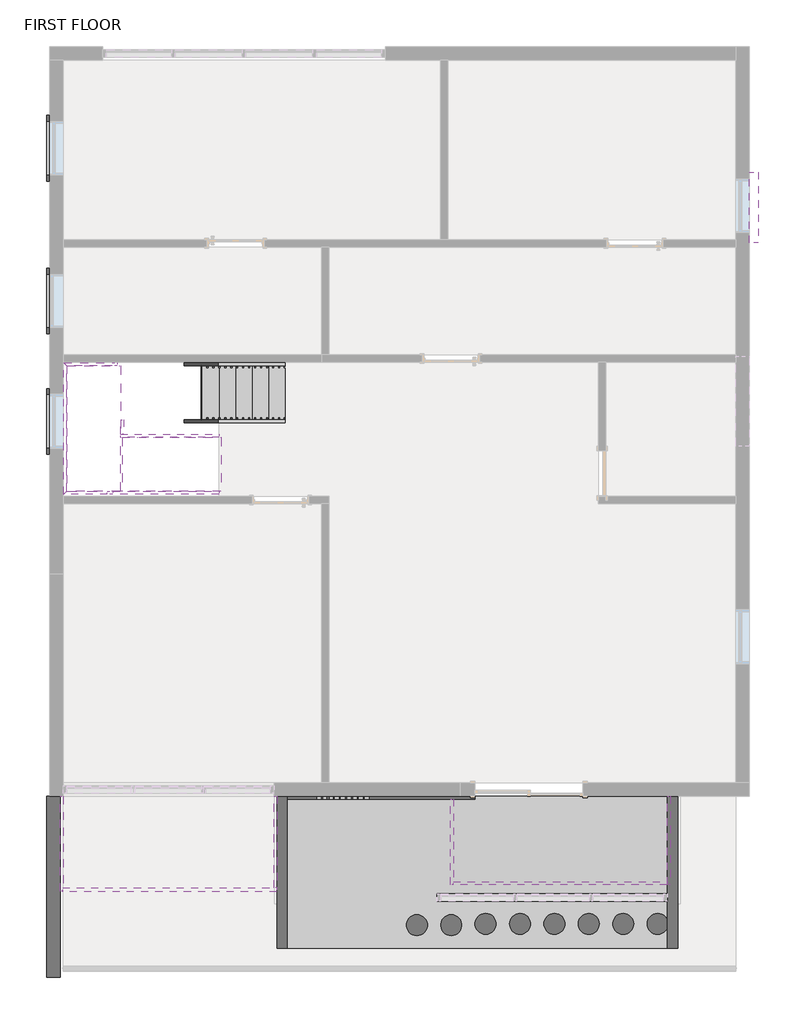
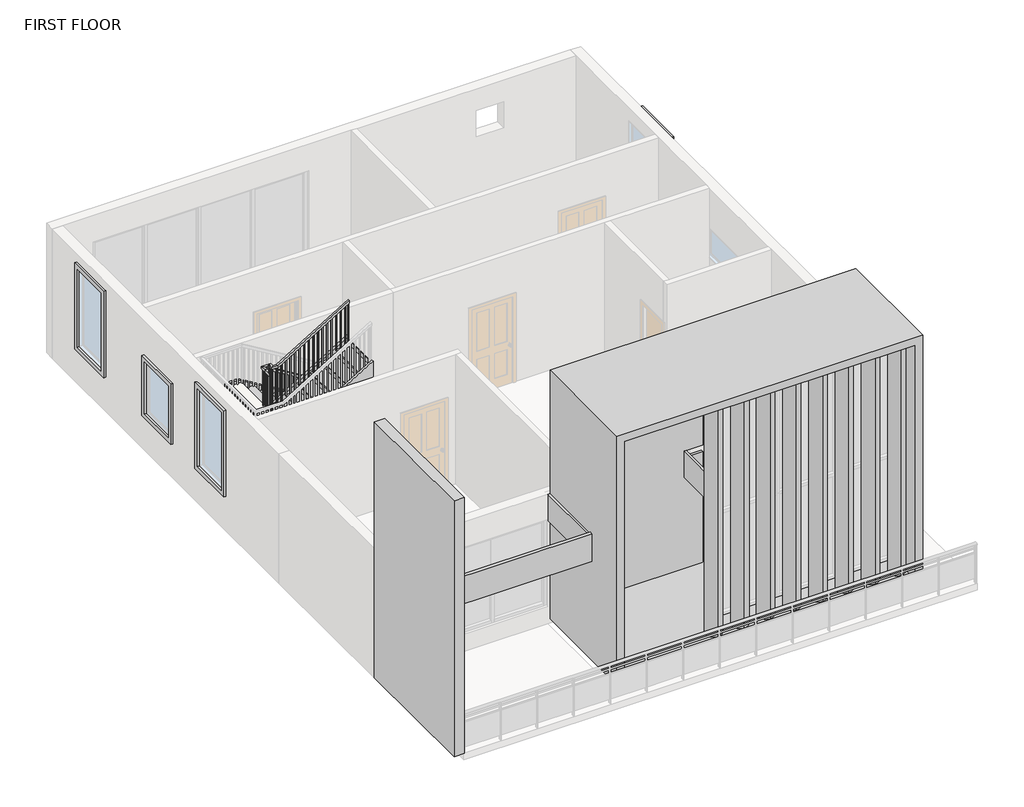
# One storey, part 4 of 4: 14 proxies, 8 members, 2 stair flights, 1 railing, 1 slab.
"""IFC4 building model written with IfcOpenShell, lengths in millimetres."""

from ifc_helpers import new_model, si_unit, frame, origin, place, context, project, spatial, polyline, outline, extrude, faceted_brep, transform, mapped, element, save
from components import generic_models_10_generic_models_10_d6021447, generic_models_12_generic_models_12_b23cc652, generic_models_14_generic_models_13_4ffb657b, generic_models_2_generic_models_2_0bdea63f, generic_models_21_generic_models_23_029173b4, generic_models_24_generic_models_24_8205a677, generic_models_3_generic_models_3_c928dfbd, generic_models_4_generic_models_4_3414f660, generic_models_5_generic_models_4_8e188f4a, generic_models_6_generic_models_6_105658a1, generic_models_7_generic_models_7_cfbcc48d, generic_models_8_generic_models_8_ec4d4fb3, generic_models_9_generic_models_9_a63bbd8a, non_monolithic_landing_6f6b2bb5, stair_flight_dce79e7d, stair_flight_8dca3de9

model = new_model("IFC4")

# Units and contexts
model_context = context("Model", 3, world=origin())
ifc_project = project(units=[si_unit("LENGTHUNIT", "METRE", prefix="MILLI")], contexts=[model_context])

# Site, building, storey
site = spatial("IfcSite", under=ifc_project)
building = spatial("IfcBuilding", under=site)
storey = spatial("IfcBuildingStorey", under=building, Name="FIRST FLOOR", Elevation=3352.8)

# Proxies
placement = place(None, origin())
generic_models_10_generic_models_10_shape = generic_models_10_generic_models_10_d6021447(model_context)
element("IfcBuildingElementProxy", 1, Name="Generic Models 10 : Generic Models 10", ObjectType="Generic Models 10 : Generic Models 10", at=placement, inside=storey, context=model_context, shape_type="MappedRepresentation", body=[
    mapped(generic_models_10_generic_models_10_shape, transform((0.0, 0.0, 0.0), x_axis=(1.0, 0.0, 0.0), y_axis=(0.0, 1.0, 0.0), z_axis=(0.0, 0.0, 1.0))),
])
generic_models_12_generic_models_12_shape = generic_models_12_generic_models_12_b23cc652(model_context)
element("IfcBuildingElementProxy", 2, Name="Generic Models 12 : Generic Models 12", ObjectType="Generic Models 12 : Generic Models 12", at=placement, inside=storey, context=model_context, shape_type="MappedRepresentation", body=[
    mapped(generic_models_12_generic_models_12_shape, transform((0.0, 0.0, 0.0), x_axis=(1.0, 0.0, 0.0), y_axis=(0.0, 1.0, 0.0), z_axis=(0.0, 0.0, 1.0))),
])
generic_models_14_generic_models_13_shape = generic_models_14_generic_models_13_4ffb657b(model_context)
element("IfcBuildingElementProxy", 3, Name="Generic Models 15 : Generic Models 13", ObjectType="Generic Models 15 : Generic Models 13", at=placement, inside=storey, context=model_context, shape_type="MappedRepresentation", body=[
    mapped(generic_models_14_generic_models_13_shape, transform((0.0, 7315.2, -3048.0), x_axis=(1.0, 0.0, 0.0), y_axis=(0.0, 1.0, 0.0), z_axis=(0.0, 0.0, 1.0))),
])
generic_models_2_generic_models_2_shape = generic_models_2_generic_models_2_0bdea63f(model_context)
element("IfcBuildingElementProxy", 4, Name="Generic Models 2 : Generic Models 2", ObjectType="Generic Models 2 : Generic Models 2", at=placement, inside=storey, context=model_context, shape_type="MappedRepresentation", body=[
    mapped(generic_models_2_generic_models_2_shape, transform((0.0, 0.0, 0.0), x_axis=(1.0, 0.0, 0.0), y_axis=(0.0, 1.0, 0.0), z_axis=(0.0, 0.0, 1.0))),
])
generic_models_21_generic_models_23_shape = generic_models_21_generic_models_23_029173b4(model_context)
element("IfcBuildingElementProxy", 5, Name="Generic Models 21 : Generic Models 23", ObjectType="Generic Models 21 : Generic Models 23", at=placement, inside=storey, context=model_context, shape_type="MappedRepresentation", body=[
    mapped(generic_models_21_generic_models_23_shape, transform((0.0, 0.0, -3048.0), x_axis=(1.0, 0.0, 0.0), y_axis=(0.0, 1.0, 0.0), z_axis=(0.0, 0.0, 1.0))),
])
generic_models_24_generic_models_24_shape = generic_models_24_generic_models_24_8205a677(model_context)
element("IfcBuildingElementProxy", 6, Name="Generic Models 25 : Generic Models 24", ObjectType="Generic Models 25 : Generic Models 24", at=placement, inside=storey, context=model_context, shape_type="MappedRepresentation", body=[
    mapped(generic_models_24_generic_models_24_shape, transform((0.0, 0.0, -3048.0), x_axis=(1.0, 0.0, 0.0), y_axis=(0.0, 1.0, 0.0), z_axis=(0.0, 0.0, 1.0))),
])
element("IfcBuildingElementProxy", 7, Name="Generic Models 28 : Generic Models 23", ObjectType="Generic Models 28 : Generic Models 23", at=placement, inside=storey, context=model_context, shape_type="MappedRepresentation", body=[
    mapped(generic_models_21_generic_models_23_shape, transform((0.0, -4635.5, -3048.0), x_axis=(1.0, 0.0, 0.0), y_axis=(0.0, 1.0, 0.0), z_axis=(0.0, 0.0, 1.0))),
])
generic_models_3_generic_models_3_shape = generic_models_3_generic_models_3_c928dfbd(model_context)
element("IfcBuildingElementProxy", 8, Name="Generic Models 3 : Generic Models 3", ObjectType="Generic Models 3 : Generic Models 3", at=placement, inside=storey, context=model_context, shape_type="MappedRepresentation", body=[
    mapped(generic_models_3_generic_models_3_shape, transform((0.0, 0.0, 0.0), x_axis=(1.0, 0.0, 0.0), y_axis=(0.0, 1.0, 0.0), z_axis=(0.0, 0.0, 1.0))),
])
generic_models_4_generic_models_4_shape = generic_models_4_generic_models_4_3414f660(model_context)
element("IfcBuildingElementProxy", 9, Name="Generic Models 4 : Generic Models 4", ObjectType="Generic Models 4 : Generic Models 4", at=placement, inside=storey, context=model_context, shape_type="MappedRepresentation", body=[
    mapped(generic_models_4_generic_models_4_shape, transform((0.0, 0.0, 0.0), x_axis=(1.0, 0.0, 0.0), y_axis=(0.0, 1.0, 0.0), z_axis=(0.0, 0.0, 1.0))),
])
generic_models_5_generic_models_4_shape = generic_models_5_generic_models_4_8e188f4a(model_context)
element("IfcBuildingElementProxy", 10, Name="Generic Models 5 : Generic Models 4", ObjectType="Generic Models 5 : Generic Models 4", at=placement, inside=storey, context=model_context, shape_type="MappedRepresentation", body=[
    mapped(generic_models_5_generic_models_4_shape, transform((-6635.75, 0.0, 0.0), x_axis=(1.0, 0.0, 0.0), y_axis=(0.0, 1.0, 0.0), z_axis=(0.0, 0.0, 1.0))),
])
generic_models_6_generic_models_6_shape = generic_models_6_generic_models_6_105658a1(model_context)
element("IfcBuildingElementProxy", 11, Name="Generic Models 6 : Generic Models 6", ObjectType="Generic Models 6 : Generic Models 6", at=placement, inside=storey, context=model_context, shape_type="MappedRepresentation", body=[
    mapped(generic_models_6_generic_models_6_shape, transform((0.0, 0.0, 0.0), x_axis=(1.0, 0.0, 0.0), y_axis=(0.0, 1.0, 0.0), z_axis=(0.0, 0.0, 1.0))),
])
generic_models_7_generic_models_7_shape = generic_models_7_generic_models_7_cfbcc48d(model_context)
element("IfcBuildingElementProxy", 12, Name="Generic Models 7 : Generic Models 7", ObjectType="Generic Models 7 : Generic Models 7", at=placement, inside=storey, context=model_context, shape_type="MappedRepresentation", body=[
    mapped(generic_models_7_generic_models_7_shape, transform((0.0, 0.0, 0.0), x_axis=(1.0, 0.0, 0.0), y_axis=(0.0, 1.0, 0.0), z_axis=(0.0, 0.0, 1.0))),
])
generic_models_8_generic_models_8_shape = generic_models_8_generic_models_8_ec4d4fb3(model_context)
element("IfcBuildingElementProxy", 13, Name="Generic Models 8 : Generic Models 8", ObjectType="Generic Models 8 : Generic Models 8", at=placement, inside=storey, context=model_context, shape_type="MappedRepresentation", body=[
    mapped(generic_models_8_generic_models_8_shape, transform((0.0, 0.0, 0.0), x_axis=(1.0, 0.0, 0.0), y_axis=(0.0, 1.0, 0.0), z_axis=(0.0, 0.0, 1.0))),
])
generic_models_9_generic_models_9_shape = generic_models_9_generic_models_9_a63bbd8a(model_context)
element("IfcBuildingElementProxy", 14, Name="Generic Models 9 : Generic Models 9", ObjectType="Generic Models 9 : Generic Models 9", at=placement, inside=storey, context=model_context, shape_type="MappedRepresentation", body=[
    mapped(generic_models_9_generic_models_9_shape, transform((0.0, 0.0, 0.0), x_axis=(1.0, 0.0, 0.0), y_axis=(0.0, 1.0, 0.0), z_axis=(0.0, 0.0, 1.0))),
])

# Members
element("IfcMember", 15, ObjectType="Stringer - 2\" Width", at=placement, inside=storey, context=model_context, shape_type="SweptSolid", body=[
    extrude(outline(polyline([(3657.6, -5990.8517085), (3869.714512, -5990.8517085), (5532.2599665, -8734.0517085), (5175.851205, -8734.0517085), (3657.6, -6228.9372203), (3657.6, -5990.8517085)])), frame((0.0, 1953.8826226, 0.0), z_axis=(0.0, 1.0, 0.0), x_axis=(0.0, 0.0, 1.0)), (0.0, 0.0, 1.0), 50.8),
])
element("IfcMember", 16, ObjectType="Stringer - 2\" Width", at=placement, inside=storey, context=model_context, shape_type="SweptSolid", body=[
    extrude(outline(polyline([(3657.6, -5990.8517085), (3869.714512, -5990.8517085), (5596.4666667, -8839.9927638), (5291.6666667, -8925.1472203), (3657.6, -6228.9372203), (3657.6, -5990.8517085)])), frame((0.0, 2919.0826226, 0.0), z_axis=(0.0, 1.0, 0.0), x_axis=(0.0, 0.0, 1.0)), (0.0, 0.0, 1.0), 50.8),
])
element("IfcMember", 17, ObjectType="Stringer - 2\" Width", at=placement, inside=storey, context=model_context, shape_type="SweptSolid", body=[
    extrude(outline(polyline([(5732.3811786, -8784.8517085), (5375.9724171, -8784.8517085), (6391.9724171, -7108.4517085), (6748.3811786, -7108.4517085), (5732.3811786, -8784.8517085)])), frame((0.0, 1706.4165128, 0.0), z_axis=(0.0, 1.0, 0.0), x_axis=(0.0, 0.0, 1.0)), (0.0, 0.0, 1.0), 50.8),
])
element("IfcMember", 18, ObjectType="Stringer - 2\" Width", at=placement, inside=storey, context=model_context, shape_type="SweptSolid", body=[
    extrude(outline(polyline([(5596.4666667, -9009.1106533), (5291.6666667, -8923.9561967), (6391.9724171, -7108.4517085), (6748.3811786, -7108.4517085), (5596.4666667, -9009.1106533)])), frame((0.0, 741.2165128, 0.0), z_axis=(0.0, 1.0, 0.0), x_axis=(0.0, 0.0, 1.0)), (0.0, 0.0, 1.0), 50.8),
])
element("IfcMember", 19, ObjectType="Stringer - 2\" Width", at=placement, inside=storey, context=model_context, shape_type="SweptSolid", body=[
    extrude(outline(polyline([(-8734.0517085, 1757.2165128), (-8784.8517085, 1757.2165128), (-8784.8517085, 2004.6826226), (-8734.0517085, 2004.6826226), (-8734.0517085, 1757.2165128)])), frame((0.0, 0.0, 5291.6666667), z_axis=(0.0, 0.0, 1.0), x_axis=(1.0, 0.0, 0.0)), (0.0, 0.0, 1.0), 304.8),
])
element("IfcMember", 20, ObjectType="Stringer - 2\" Width", at=placement, inside=storey, context=model_context, shape_type="Brep", body=[
    faceted_brep([(-8839.9927638, 2919.0826226, 5596.4666667), (-8839.9927638, 2969.8826226, 5596.4666667), (-9750.0517085, 2969.8826226, 5596.4666667), (-9699.2517085, 2919.0826226, 5596.4666667), (-8925.1472203, 2919.0826226, 5291.6666667), (-9699.2517085, 2919.0826226, 5291.6666667), (-8925.1472203, 2969.8826226, 5291.6666667), (-9750.0517085, 2969.8826226, 5291.6666667)], [[[0, 1, 2, 3]], [[4, 0, 3, 5]], [[6, 4, 5, 7]], [[1, 6, 7, 2]], [[1, 0, 4, 6]], [[2, 7, 5, 3]]]),
])
element("IfcMember", 21, ObjectType="Stringer - 2\" Width", at=placement, inside=storey, context=model_context, shape_type="SweptSolid", body=[
    extrude(outline(polyline([(-9750.0517085, 2969.8826226), (-9699.2517085, 2919.0826226), (-9699.2517085, 792.0165128), (-9750.0517085, 741.2165128), (-9750.0517085, 2969.8826226)])), frame((0.0, 0.0, 5291.6666667), z_axis=(0.0, 0.0, 1.0), x_axis=(1.0, 0.0, 0.0)), (0.0, 0.0, 1.0), 304.8),
])
element("IfcMember", 22, ObjectType="Stringer - 2\" Width", at=placement, inside=storey, context=model_context, shape_type="Brep", body=[
    faceted_brep([(-9699.2517085, 792.0165128, 5596.4666667), (-9750.0517085, 741.2165128, 5596.4666667), (-9009.1106533, 741.2165128, 5596.4666667), (-9009.1106533, 792.0165128, 5596.4666667), (-9699.2517085, 792.0165128, 5291.6666667), (-8923.9561967, 792.0165128, 5291.6666667), (-9750.0517085, 741.2165128, 5291.6666667), (-8923.9561967, 741.2165128, 5291.6666667)], [[[0, 1, 2, 3]], [[4, 0, 3, 5]], [[6, 4, 5, 7]], [[1, 6, 7, 2]], [[1, 0, 4, 6]], [[2, 7, 5, 3]]]),
])

# Railing
element("IfcRailing", 23, ObjectType="Handrail - Rectangular", at=placement, inside=storey, context=model_context, shape_type="SolidModel", body=[
    faceted_brep([(-5990.8517085, 2004.6826226, 4741.3333333), (-5990.8517085, 2004.6826226, 4681.9318731), (-5990.8517085, 2055.4826226, 4681.9318731), (-5990.8517085, 2055.4826226, 4741.3333333), (-8708.6517085, 2004.6826226, 6388.4848485), (-8759.4517085, 2004.6826226, 6359.871267), (-8759.4517085, 2055.4826226, 6359.871267), (-8708.6517085, 2055.4826226, 6388.4848485), (-8708.6517085, 2004.6826226, 6434.6666667), (-8759.4517085, 2004.6826226, 6383.8666667), (-8759.4517085, 2055.4826226, 6383.8666667), (-8708.6517085, 2055.4826226, 6434.6666667), (-8784.8517085, 2004.6826226, 6434.6666667), (-8784.8517085, 2004.6826226, 6383.8666667), (-8835.6517085, 2055.4826226, 6383.8666667), (-8835.6517085, 2055.4826226, 6434.6666667), (-8784.8517085, 1928.4826226, 6434.6666667), (-8784.8517085, 1928.4826226, 6383.8666667), (-8835.6517085, 1928.4826226, 6383.8666667), (-8835.6517085, 1928.4826226, 6434.6666667), (-8784.8517085, 1782.6165128, 6434.6666667), (-8784.8517085, 1731.8165128, 6383.8666667), (-8835.6517085, 1731.8165128, 6383.8666667), (-8835.6517085, 1782.6165128, 6434.6666667), (-8784.8517085, 1782.6165128, 6650.1818182), (-8784.8517085, 1731.8165128, 6599.3818182), (-8835.6517085, 1731.8165128, 6599.3818182), (-8835.6517085, 1782.6165128, 6650.1818182), (-8784.8517085, 1706.4165128, 6650.1818182), (-8784.8517085, 1706.4165128, 6599.3818182), (-8835.6517085, 1655.6165128, 6599.3818182), (-8835.6517085, 1655.6165128, 6650.1818182), (-8708.6517085, 1706.4165128, 6650.1818182), (-8694.4592991, 1706.4165128, 6599.3818182), (-8694.4592991, 1655.6165128, 6599.3818182), (-8708.6517085, 1655.6165128, 6650.1818182), (-7108.4517085, 1706.4165128, 7620.0), (-7108.4517085, 1655.6165128, 7620.0), (-7108.4517085, 1655.6165128, 7560.5985397), (-7108.4517085, 1706.4165128, 7560.5985397)], [[[0, 1, 2, 3]], [[1, 0, 4, 5]], [[2, 1, 5, 6]], [[3, 2, 6, 7]], [[0, 3, 7, 4]], [[5, 4, 8, 9]], [[6, 5, 9, 10]], [[7, 6, 10, 11]], [[4, 7, 11, 8]], [[9, 8, 12, 13]], [[10, 9, 13, 14]], [[11, 10, 14, 15]], [[8, 11, 15, 12]], [[13, 12, 16, 17]], [[14, 13, 17, 18]], [[15, 14, 18, 19]], [[12, 15, 19, 16]], [[17, 16, 20, 21]], [[18, 17, 21, 22]], [[19, 18, 22, 23]], [[16, 19, 23, 20]], [[21, 20, 24, 25]], [[22, 21, 25, 26]], [[23, 22, 26, 27]], [[20, 23, 27, 24]], [[25, 24, 28, 29]], [[26, 25, 29, 30]], [[27, 26, 30, 31]], [[24, 27, 31, 28]], [[29, 28, 32, 33]], [[30, 29, 33, 34]], [[31, 30, 34, 35]], [[28, 31, 35, 32]], [[36, 37, 38, 39]], [[33, 32, 36, 39]], [[34, 33, 39, 38]], [[35, 34, 38, 37]], [[32, 35, 37, 36]]]),
    extrude(outline(polyline([(7508.6439943, -7194.1767085), (6536.2666667, -7194.1767085), (6536.2666667, -7175.1267085), (7520.1894488, -7175.1267085), (7508.6439943, -7194.1767085)])), frame((0.0, 1671.4915128, 0.0), z_axis=(0.0, 1.0, 0.0), x_axis=(0.0, 0.0, 1.0)), (0.0, 0.0, 1.0), 19.05),
    extrude(outline(polyline([(7447.0682367, -7295.7767085), (6536.2666667, -7295.7767085), (6536.2666667, -7276.7267085), (7458.6136913, -7276.7267085), (7447.0682367, -7295.7767085)])), frame((0.0, 1671.4915128, 0.0), z_axis=(0.0, 1.0, 0.0), x_axis=(0.0, 0.0, 1.0)), (0.0, 0.0, 1.0), 19.05),
    extrude(outline(polyline([(7385.4924791, -7397.3767085), (6536.2666667, -7397.3767085), (6536.2666667, -7378.3267085), (7397.0379337, -7378.3267085), (7385.4924791, -7397.3767085)])), frame((0.0, 1671.4915128, 0.0), z_axis=(0.0, 1.0, 0.0), x_axis=(0.0, 0.0, 1.0)), (0.0, 0.0, 1.0), 19.05),
    extrude(outline(polyline([(7323.9167216, -7498.9767085), (6366.9333333, -7498.9767085), (6366.9333333, -7479.9267085), (7335.4621761, -7479.9267085), (7323.9167216, -7498.9767085)])), frame((0.0, 1671.4915128, 0.0), z_axis=(0.0, 1.0, 0.0), x_axis=(0.0, 0.0, 1.0)), (0.0, 0.0, 1.0), 19.05),
    extrude(outline(polyline([(7262.340964, -7600.5767085), (6366.9333333, -7600.5767085), (6366.9333333, -7581.5267085), (7273.8864185, -7581.5267085), (7262.340964, -7600.5767085)])), frame((0.0, 1671.4915128, 0.0), z_axis=(0.0, 1.0, 0.0), x_axis=(0.0, 0.0, 1.0)), (0.0, 0.0, 1.0), 19.05),
    extrude(outline(polyline([(7200.7652064, -7702.1767085), (6197.6, -7702.1767085), (6197.6, -7683.1267085), (7212.310661, -7683.1267085), (7200.7652064, -7702.1767085)])), frame((0.0, 1671.4915128, 0.0), z_axis=(0.0, 1.0, 0.0), x_axis=(0.0, 0.0, 1.0)), (0.0, 0.0, 1.0), 19.05),
    extrude(outline(polyline([(7139.1894488, -7803.7767085), (6197.6, -7803.7767085), (6197.6, -7784.7267085), (7150.7349034, -7784.7267085), (7139.1894488, -7803.7767085)])), frame((0.0, 1671.4915128, 0.0), z_axis=(0.0, 1.0, 0.0), x_axis=(0.0, 0.0, 1.0)), (0.0, 0.0, 1.0), 19.05),
    extrude(outline(polyline([(7077.6136913, -7905.3767085), (6197.6, -7905.3767085), (6197.6, -7886.3267085), (7089.1591458, -7886.3267085), (7077.6136913, -7905.3767085)])), frame((0.0, 1671.4915128, 0.0), z_axis=(0.0, 1.0, 0.0), x_axis=(0.0, 0.0, 1.0)), (0.0, 0.0, 1.0), 19.05),
    extrude(outline(polyline([(7016.0379337, -8006.9767085), (6028.2666667, -8006.9767085), (6028.2666667, -7987.9267085), (7027.5833882, -7987.9267085), (7016.0379337, -8006.9767085)])), frame((0.0, 1671.4915128, 0.0), z_axis=(0.0, 1.0, 0.0), x_axis=(0.0, 0.0, 1.0)), (0.0, 0.0, 1.0), 19.05),
    extrude(outline(polyline([(6954.4621761, -8108.5767085), (6028.2666667, -8108.5767085), (6028.2666667, -8089.5267085), (6966.0076307, -8089.5267085), (6954.4621761, -8108.5767085)])), frame((0.0, 1671.4915128, 0.0), z_axis=(0.0, 1.0, 0.0), x_axis=(0.0, 0.0, 1.0)), (0.0, 0.0, 1.0), 19.05),
    extrude(outline(polyline([(6892.8864185, -8210.1767085), (6028.2666667, -8210.1767085), (6028.2666667, -8191.1267085), (6904.4318731, -8191.1267085), (6892.8864185, -8210.1767085)])), frame((0.0, 1671.4915128, 0.0), z_axis=(0.0, 1.0, 0.0), x_axis=(0.0, 0.0, 1.0)), (0.0, 0.0, 1.0), 19.05),
    extrude(outline(polyline([(6831.310661, -8311.7767085), (5858.9333333, -8311.7767085), (5858.9333333, -8292.7267085), (6842.8561155, -8292.7267085), (6831.310661, -8311.7767085)])), frame((0.0, 1671.4915128, 0.0), z_axis=(0.0, 1.0, 0.0), x_axis=(0.0, 0.0, 1.0)), (0.0, 0.0, 1.0), 19.05),
    extrude(outline(polyline([(6769.7349034, -8413.3767085), (5858.9333333, -8413.3767085), (5858.9333333, -8394.3267085), (6781.2803579, -8394.3267085), (6769.7349034, -8413.3767085)])), frame((0.0, 1671.4915128, 0.0), z_axis=(0.0, 1.0, 0.0), x_axis=(0.0, 0.0, 1.0)), (0.0, 0.0, 1.0), 19.05),
    extrude(outline(polyline([(6708.1591458, -8514.9767085), (5858.9333333, -8514.9767085), (5858.9333333, -8495.9267085), (6719.7046004, -8495.9267085), (6708.1591458, -8514.9767085)])), frame((0.0, 1671.4915128, 0.0), z_axis=(0.0, 1.0, 0.0), x_axis=(0.0, 0.0, 1.0)), (0.0, 0.0, 1.0), 19.05),
    extrude(outline(polyline([(6646.5833882, -8616.5767085), (5689.6, -8616.5767085), (5689.6, -8597.5267085), (6658.1288428, -8597.5267085), (6646.5833882, -8616.5767085)])), frame((0.0, 1671.4915128, 0.0), z_axis=(0.0, 1.0, 0.0), x_axis=(0.0, 0.0, 1.0)), (0.0, 0.0, 1.0), 19.05),
    extrude(outline(polyline([(6585.0076307, -8718.1767085), (5689.6, -8718.1767085), (5689.6, -8699.1267085), (6596.5530852, -8699.1267085), (6585.0076307, -8718.1767085)])), frame((0.0, 1671.4915128, 0.0), z_axis=(0.0, 1.0, 0.0), x_axis=(0.0, 0.0, 1.0)), (0.0, 0.0, 1.0), 19.05),
    extrude(outline(polyline([(-8800.7267085, 1734.8076226), (-8800.7267085, 1715.7576226), (-8819.7767085, 1715.7576226), (-8819.7767085, 1734.8076226), (-8800.7267085, 1734.8076226)])), frame((0.0, 0.0, 5520.2666667), z_axis=(0.0, 0.0, 1.0), x_axis=(1.0, 0.0, 0.0)), (0.0, 0.0, 1.0), 1079.1151515),
    extrude(outline(polyline([(-8800.7267085, 1836.4076226), (-8800.7267085, 1817.3576226), (-8819.7767085, 1817.3576226), (-8819.7767085, 1836.4076226), (-8800.7267085, 1836.4076226)])), frame((0.0, 0.0, 5520.2666667), z_axis=(0.0, 0.0, 1.0), x_axis=(1.0, 0.0, 0.0)), (0.0, 0.0, 1.0), 863.6),
    extrude(outline(polyline([(-8800.7267085, 1938.0076226), (-8800.7267085, 1918.9576226), (-8819.7767085, 1918.9576226), (-8819.7767085, 1938.0076226), (-8800.7267085, 1938.0076226)])), frame((0.0, 0.0, 5520.2666667), z_axis=(0.0, 0.0, 1.0), x_axis=(1.0, 0.0, 0.0)), (0.0, 0.0, 1.0), 863.6),
    extrude(outline(polyline([(-8724.5267085, 2020.5576226), (-8743.5767085, 2020.5576226), (-8743.5767085, 2039.6076226), (-8724.5267085, 2039.6076226), (-8724.5267085, 2020.5576226)])), frame((0.0, 0.0, 5350.9333333), z_axis=(0.0, 0.0, 1.0), x_axis=(1.0, 0.0, 0.0)), (0.0, 0.0, 1.0), 1032.9333333),
    extrude(outline(polyline([(6288.6742973, -8641.9767085), (5350.9333333, -8641.9767085), (5350.9333333, -8622.9267085), (6277.1288428, -8622.9267085), (6288.6742973, -8641.9767085)])), frame((0.0, 2020.5576226, 0.0), z_axis=(0.0, 1.0, 0.0), x_axis=(0.0, 0.0, 1.0)), (0.0, 0.0, 1.0), 19.05),
    extrude(outline(polyline([(6227.0985397, -8540.3767085), (5350.9333333, -8540.3767085), (5350.9333333, -8521.3267085), (6215.5530852, -8521.3267085), (6227.0985397, -8540.3767085)])), frame((0.0, 2020.5576226, 0.0), z_axis=(0.0, 1.0, 0.0), x_axis=(0.0, 0.0, 1.0)), (0.0, 0.0, 1.0), 19.05),
    extrude(outline(polyline([(6165.5227822, -8438.7767085), (5181.6, -8438.7767085), (5181.6, -8419.7267085), (6153.9773276, -8419.7267085), (6165.5227822, -8438.7767085)])), frame((0.0, 2020.5576226, 0.0), z_axis=(0.0, 1.0, 0.0), x_axis=(0.0, 0.0, 1.0)), (0.0, 0.0, 1.0), 19.05),
    extrude(outline(polyline([(6103.9470246, -8337.1767085), (5181.6, -8337.1767085), (5181.6, -8318.1267085), (6092.40157, -8318.1267085), (6103.9470246, -8337.1767085)])), frame((0.0, 2020.5576226, 0.0), z_axis=(0.0, 1.0, 0.0), x_axis=(0.0, 0.0, 1.0)), (0.0, 0.0, 1.0), 19.05),
    extrude(outline(polyline([(6042.371267, -8235.5767085), (5181.6, -8235.5767085), (5181.6, -8216.5267085), (6030.8258125, -8216.5267085), (6042.371267, -8235.5767085)])), frame((0.0, 2020.5576226, 0.0), z_axis=(0.0, 1.0, 0.0), x_axis=(0.0, 0.0, 1.0)), (0.0, 0.0, 1.0), 19.05),
    extrude(outline(polyline([(5980.7955094, -8133.9767085), (5012.2666667, -8133.9767085), (5012.2666667, -8114.9267085), (5969.2500549, -8114.9267085), (5980.7955094, -8133.9767085)])), frame((0.0, 2020.5576226, 0.0), z_axis=(0.0, 1.0, 0.0), x_axis=(0.0, 0.0, 1.0)), (0.0, 0.0, 1.0), 19.05),
    extrude(outline(polyline([(5919.2197519, -8032.3767085), (5012.2666667, -8032.3767085), (5012.2666667, -8013.3267085), (5907.6742973, -8013.3267085), (5919.2197519, -8032.3767085)])), frame((0.0, 2020.5576226, 0.0), z_axis=(0.0, 1.0, 0.0), x_axis=(0.0, 0.0, 1.0)), (0.0, 0.0, 1.0), 19.05),
    extrude(outline(polyline([(5857.6439943, -7930.7767085), (4842.9333333, -7930.7767085), (4842.9333333, -7911.7267085), (5846.0985397, -7911.7267085), (5857.6439943, -7930.7767085)])), frame((0.0, 2020.5576226, 0.0), z_axis=(0.0, 1.0, 0.0), x_axis=(0.0, 0.0, 1.0)), (0.0, 0.0, 1.0), 19.05),
    extrude(outline(polyline([(5796.0682367, -7829.1767085), (4842.9333333, -7829.1767085), (4842.9333333, -7810.1267085), (5784.5227822, -7810.1267085), (5796.0682367, -7829.1767085)])), frame((0.0, 2020.5576226, 0.0), z_axis=(0.0, 1.0, 0.0), x_axis=(0.0, 0.0, 1.0)), (0.0, 0.0, 1.0), 19.05),
    extrude(outline(polyline([(5734.4924791, -7727.5767085), (4842.9333333, -7727.5767085), (4842.9333333, -7708.5267085), (5722.9470246, -7708.5267085), (5734.4924791, -7727.5767085)])), frame((0.0, 2020.5576226, 0.0), z_axis=(0.0, 1.0, 0.0), x_axis=(0.0, 0.0, 1.0)), (0.0, 0.0, 1.0), 19.05),
    extrude(outline(polyline([(5672.9167216, -7625.9767085), (4673.6, -7625.9767085), (4673.6, -7606.9267085), (5661.371267, -7606.9267085), (5672.9167216, -7625.9767085)])), frame((0.0, 2020.5576226, 0.0), z_axis=(0.0, 1.0, 0.0), x_axis=(0.0, 0.0, 1.0)), (0.0, 0.0, 1.0), 19.05),
    extrude(outline(polyline([(5611.340964, -7524.3767085), (4673.6, -7524.3767085), (4673.6, -7505.3267085), (5599.7955094, -7505.3267085), (5611.340964, -7524.3767085)])), frame((0.0, 2020.5576226, 0.0), z_axis=(0.0, 1.0, 0.0), x_axis=(0.0, 0.0, 1.0)), (0.0, 0.0, 1.0), 19.05),
    extrude(outline(polyline([(5549.7652064, -7422.7767085), (4673.6, -7422.7767085), (4673.6, -7403.7267085), (5538.2197519, -7403.7267085), (5549.7652064, -7422.7767085)])), frame((0.0, 2020.5576226, 0.0), z_axis=(0.0, 1.0, 0.0), x_axis=(0.0, 0.0, 1.0)), (0.0, 0.0, 1.0), 19.05),
    extrude(outline(polyline([(5488.1894488, -7321.1767085), (4504.2666667, -7321.1767085), (4504.2666667, -7302.1267085), (5476.6439943, -7302.1267085), (5488.1894488, -7321.1767085)])), frame((0.0, 2020.5576226, 0.0), z_axis=(0.0, 1.0, 0.0), x_axis=(0.0, 0.0, 1.0)), (0.0, 0.0, 1.0), 19.05),
    extrude(outline(polyline([(5426.6136913, -7219.5767085), (4504.2666667, -7219.5767085), (4504.2666667, -7200.5267085), (5415.0682367, -7200.5267085), (5426.6136913, -7219.5767085)])), frame((0.0, 2020.5576226, 0.0), z_axis=(0.0, 1.0, 0.0), x_axis=(0.0, 0.0, 1.0)), (0.0, 0.0, 1.0), 19.05),
    extrude(outline(polyline([(5365.0379337, -7117.9767085), (4504.2666667, -7117.9767085), (4504.2666667, -7098.9267085), (5353.4924791, -7098.9267085), (5365.0379337, -7117.9767085)])), frame((0.0, 2020.5576226, 0.0), z_axis=(0.0, 1.0, 0.0), x_axis=(0.0, 0.0, 1.0)), (0.0, 0.0, 1.0), 19.05),
    extrude(outline(polyline([(5303.4621761, -7016.3767085), (4334.9333333, -7016.3767085), (4334.9333333, -6997.3267085), (5291.9167216, -6997.3267085), (5303.4621761, -7016.3767085)])), frame((0.0, 2020.5576226, 0.0), z_axis=(0.0, 1.0, 0.0), x_axis=(0.0, 0.0, 1.0)), (0.0, 0.0, 1.0), 19.05),
    extrude(outline(polyline([(5241.8864185, -6914.7767085), (4334.9333333, -6914.7767085), (4334.9333333, -6895.7267085), (5230.340964, -6895.7267085), (5241.8864185, -6914.7767085)])), frame((0.0, 2020.5576226, 0.0), z_axis=(0.0, 1.0, 0.0), x_axis=(0.0, 0.0, 1.0)), (0.0, 0.0, 1.0), 19.05),
    extrude(outline(polyline([(5180.310661, -6813.1767085), (4165.6, -6813.1767085), (4165.6, -6794.1267085), (5168.7652064, -6794.1267085), (5180.310661, -6813.1767085)])), frame((0.0, 2020.5576226, 0.0), z_axis=(0.0, 1.0, 0.0), x_axis=(0.0, 0.0, 1.0)), (0.0, 0.0, 1.0), 19.05),
    extrude(outline(polyline([(5118.7349034, -6711.5767085), (4165.6, -6711.5767085), (4165.6, -6692.5267085), (5107.1894488, -6692.5267085), (5118.7349034, -6711.5767085)])), frame((0.0, 2020.5576226, 0.0), z_axis=(0.0, 1.0, 0.0), x_axis=(0.0, 0.0, 1.0)), (0.0, 0.0, 1.0), 19.05),
    extrude(outline(polyline([(5057.1591458, -6609.9767085), (4165.6, -6609.9767085), (4165.6, -6590.9267085), (5045.6136913, -6590.9267085), (5057.1591458, -6609.9767085)])), frame((0.0, 2020.5576226, 0.0), z_axis=(0.0, 1.0, 0.0), x_axis=(0.0, 0.0, 1.0)), (0.0, 0.0, 1.0), 19.05),
    extrude(outline(polyline([(4995.5833882, -6508.3767085), (3996.2666667, -6508.3767085), (3996.2666667, -6489.3267085), (4984.0379337, -6489.3267085), (4995.5833882, -6508.3767085)])), frame((0.0, 2020.5576226, 0.0), z_axis=(0.0, 1.0, 0.0), x_axis=(0.0, 0.0, 1.0)), (0.0, 0.0, 1.0), 19.05),
    extrude(outline(polyline([(4934.0076307, -6406.7767085), (3996.2666667, -6406.7767085), (3996.2666667, -6387.7267085), (4922.4621761, -6387.7267085), (4934.0076307, -6406.7767085)])), frame((0.0, 2020.5576226, 0.0), z_axis=(0.0, 1.0, 0.0), x_axis=(0.0, 0.0, 1.0)), (0.0, 0.0, 1.0), 19.05),
    extrude(outline(polyline([(4872.4318731, -6305.1767085), (3996.2666667, -6305.1767085), (3996.2666667, -6286.1267085), (4860.8864185, -6286.1267085), (4872.4318731, -6305.1767085)])), frame((0.0, 2020.5576226, 0.0), z_axis=(0.0, 1.0, 0.0), x_axis=(0.0, 0.0, 1.0)), (0.0, 0.0, 1.0), 19.05),
    extrude(outline(polyline([(4810.8561155, -6203.5767085), (3826.9333333, -6203.5767085), (3826.9333333, -6184.5267085), (4799.310661, -6184.5267085), (4810.8561155, -6203.5767085)])), frame((0.0, 2020.5576226, 0.0), z_axis=(0.0, 1.0, 0.0), x_axis=(0.0, 0.0, 1.0)), (0.0, 0.0, 1.0), 19.05),
    extrude(outline(polyline([(4749.2803579, -6101.9767085), (3826.9333333, -6101.9767085), (3826.9333333, -6082.9267085), (4737.7349034, -6082.9267085), (4749.2803579, -6101.9767085)])), frame((0.0, 2020.5576226, 0.0), z_axis=(0.0, 1.0, 0.0), x_axis=(0.0, 0.0, 1.0)), (0.0, 0.0, 1.0), 19.05),
    extrude(outline(polyline([(-8800.7267085, 1690.5415128), (-8800.7267085, 1671.4915128), (-8819.7767085, 1671.4915128), (-8819.7767085, 1690.5415128), (-8800.7267085, 1690.5415128)])), frame((0.0, 0.0, 5520.2666667), z_axis=(0.0, 0.0, 1.0), x_axis=(1.0, 0.0, 0.0)), (0.0, 0.0, 1.0), 1079.1151515),
    extrude(outline(polyline([(-8800.7267085, 2020.5576226), (-8819.7767085, 2020.5576226), (-8819.7767085, 2039.6076226), (-8800.7267085, 2039.6076226), (-8800.7267085, 2020.5576226)])), frame((0.0, 0.0, 5520.2666667), z_axis=(0.0, 0.0, 1.0), x_axis=(1.0, 0.0, 0.0)), (0.0, 0.0, 1.0), 863.6),
    extrude(outline(polyline([(7549.0530852, -7127.5017085), (6536.2666667, -7127.5017085), (6536.2666667, -7108.4517085), (7560.5985397, -7108.4517085), (7549.0530852, -7127.5017085)])), frame((0.0, 1671.4915128, 0.0), z_axis=(0.0, 1.0, 0.0), x_axis=(0.0, 0.0, 1.0)), (0.0, 0.0, 1.0), 19.05),
    extrude(outline(polyline([(4693.4773276, -6009.9017085), (3826.9333333, -6009.9017085), (3826.9333333, -5990.8517085), (4681.9318731, -5990.8517085), (4693.4773276, -6009.9017085)])), frame((0.0, 2020.5576226, 0.0), z_axis=(0.0, 1.0, 0.0), x_axis=(0.0, 0.0, 1.0)), (0.0, 0.0, 1.0), 19.05),
])

# Slab
non_monolithic_landing_shape = non_monolithic_landing_6f6b2bb5(model_context)
element("IfcSlab", 24, ObjectType="Non-Monolithic Landing", at=placement, inside=storey, context=model_context, shape_type="MappedRepresentation", body=[
    mapped(non_monolithic_landing_shape, transform((0.0, 0.0, 0.0), x_axis=(1.0, 0.0, 0.0), y_axis=(0.0, 1.0, 0.0), z_axis=(0.0, 0.0, 1.0))),
])

# Stair flights
stair_flight_shape = stair_flight_dce79e7d(model_context)
element("IfcStairFlight", 25, ObjectType="2\" Tread 1\" Nosing 1/4\" Riser", at=placement, inside=storey, context=model_context, shape_type="MappedRepresentation", body=[
    mapped(stair_flight_shape, transform((0.0, 0.0, 0.0), x_axis=(1.0, 0.0, 0.0), y_axis=(0.0, 1.0, 0.0), z_axis=(0.0, 0.0, 1.0))),
])
stair_flight_2_shape = stair_flight_8dca3de9(model_context)
element("IfcStairFlight", 26, ObjectType="2\" Tread 1\" Nosing 1/4\" Riser", at=placement, inside=storey, context=model_context, shape_type="MappedRepresentation", body=[
    mapped(stair_flight_2_shape, transform((0.0, 0.0, 0.0), x_axis=(1.0, 0.0, 0.0), y_axis=(0.0, 1.0, 0.0), z_axis=(0.0, 0.0, 1.0))),
])

save(model, "model.ifc")

# Revit data of these elements
# Type "Handrail - Rectangular"
#   Assembly Code = "C2010400"
#   built-in parameter 1008612 = 0.0416667 (stored number, unit not read)
#   built-in parameter 1008611 = 0.0416667 (stored number, unit not read)
#   built-in parameter 1008609 = 0.333333 (stored number, unit not read)
#   built-in parameter 1008604 = 0.166667 (stored number, unit not read)
#   built-in parameter 1008603 = 0.166667 (stored number, unit not read)
#   Railing Height = 3' - 0"
#   built-in parameter 1008630 = 2
#   built-in parameter 1008610 = 2
#   built-in parameter 1008618 = Baluster - Square : 3/4"
# Element 1 (IfcBuildingElementProxy, "Generic Models 10 : Generic Models 10")
#   Phase Created = New Construction
#   Materials on its faces: "WOODEN SLAT"
# Element 2 (IfcBuildingElementProxy, "Generic Models 12 : Generic Models 12")
#   Phase Created = New Construction
#   Materials on its faces: "WALL PAINT"
# Element 3 (IfcBuildingElementProxy, "Generic Models 15 : Generic Models 13")
#   Phase Created = New Construction
# Element 4 (IfcBuildingElementProxy, "Generic Models 2 : Generic Models 2")
#   Phase Created = New Construction
# Element 5 (IfcBuildingElementProxy, "Generic Models 21 : Generic Models 23")
#   Phase Created = New Construction
# Element 6 (IfcBuildingElementProxy, "Generic Models 25 : Generic Models 24")
#   Phase Created = New Construction
# Element 7 (IfcBuildingElementProxy, "Generic Models 28 : Generic Models 23")
#   Phase Created = New Construction
# Element 8 (IfcBuildingElementProxy, "Generic Models 3 : Generic Models 3")
#   Phase Created = New Construction
# Element 9 (IfcBuildingElementProxy, "Generic Models 4 : Generic Models 4")
#   Phase Created = New Construction
# Element 10 (IfcBuildingElementProxy, "Generic Models 5 : Generic Models 4")
#   Phase Created = New Construction
# Element 11 (IfcBuildingElementProxy, "Generic Models 6 : Generic Models 6")
#   Phase Created = New Construction
# Element 12 (IfcBuildingElementProxy, "Generic Models 7 : Generic Models 7")
#   Phase Created = New Construction
# Element 13 (IfcBuildingElementProxy, "Generic Models 8 : Generic Models 8")
#   Phase Created = New Construction
# Element 14 (IfcBuildingElementProxy, "Generic Models 9 : Generic Models 9")
#   Phase Created = New Construction
# Elements 15, 16, 17, 18, 19, 20, 21, 22 (IfcMember, "Stringer - 2\" Width")
#   Phase Created = New Construction
# Element 23 (IfcRailing, "Handrail - Rectangular")
#   Phase Created = New Construction
# Element 24 (IfcSlab, "Non-Monolithic Landing")
#   Phase Created = New Construction
# Elements 25, 26 (IfcStairFlight, "2\" Tread 1\" Nosing 1/4\" Riser")
#   Phase Created = New Construction
# Materials
#   "WOODEN SLAT": class "Generic", colour RGB 120 120 120, transparency 0, Cost = 0
#   "WALL PAINT": class "Generic", colour RGB 120 120 120, transparency 0, Cost = 0
